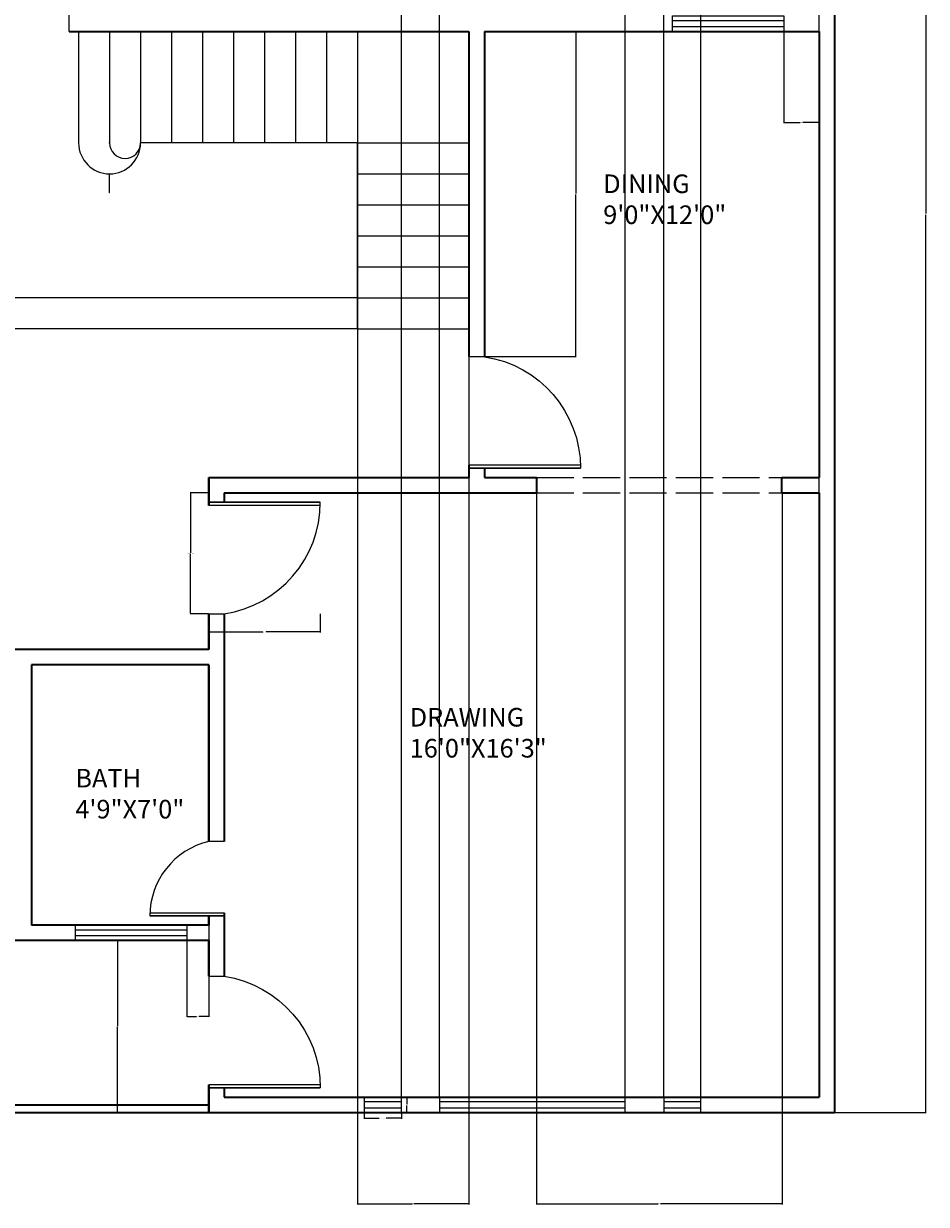
# Model space of a CAD drawing. Units: inches. Extents: x 40921 to 41493, y 89872 to 90511.
# Tile 3 of 4: x 41201 to 41493, y 89872 to 90253. Entities that reach past the tile are written whole.
import ezdxf

# ---------------------------------------------------------------- set-up
doc = ezdxf.new("R2010")
doc.units = ezdxf.units.IN
doc.header["$MEASUREMENT"] = 0
doc.linetypes.add('ACAD_ISO02W100', pattern=[15, 12, -3])
for name, color, linetype, lineweight in [('A-ANNO-DIMS', 2, 'Continuous', 18), ('A-AREA-IDEN', 7, 'Continuous', 18), ('A-DOOR', 3, 'Continuous', 20), ('A-FLOR-STRS', 7, 'Continuous', 18), ('A-GLAZ', 4, 'Continuous', 18), ('A-WALL', 7, 'Continuous', 35), ('A-WALL-OVHD', 8, 'ACAD_ISO02W100', 13)]:
    doc.layers.add(name, color=color, linetype=linetype, lineweight=lineweight)
doc.styles.get("Standard").update_dxf_attribs({"font": 'arial.ttf'})
doc.dimstyles.get("Standard").update_dxf_attribs({"dimtxt": 0.18, "dimasz": 0.18, "dimexe": 0.18, "dimexo": 0.0625, "dimgap": 0.09, "dimtad": 0, "dimtih": 1, "dimtoh": 1, "dimdec": 4, "dimzin": 0, "dimdsep": 46, "dimtxsty": 'Standard', "dimcen": 0.09, "dimadec": 0, "dimazin": 0, "dimtfac": 1, "dimtdec": 4, "dimtofl": 0, "dimtmove": 0, "dimatfit": 3, "dimfxl": 1, "dimtolj": 1, "dimtzin": 0, "dimarcsym": 0})

# ---------------------------------------------------------------- blocks, each defined once
blk = doc.blocks.new('DOOR-SWING-24IN')
for p, q in [((3, 0), (3, 24)), ((3, 24), (3, 0)), ((4, 24), (4, 0)), ((27, 0), (27, 5)), ((0, 0), (3, 0)), ((3, 0), (4, 0))]:
    blk.add_line(p, q)
blk.add_arc((3, -0.66), 24.66, 13.265, 90)
blk = doc.blocks.new('DOOR-SWING-36IN')
for p, q in [((3, 0), (3, 36)), ((3, 36), (3, 0)), ((4, 36), (4, 0)), ((39, 0), (39, 5)), ((0, 0), (3, 0)), ((3, 0), (4, 0))]:
    blk.add_line(p, q)
blk.add_arc((3, -0.4), 36.4, 8.5358, 90)
blk = doc.blocks.new('WIN-36IN')
for p, q in [((0, 36), (5, 36)), ((0, 0), (0, 36)), ((1.5, 0), (1.5, 36)), ((3.5, 36), (3.5, 0)), ((5, 36), (5, 0)), ((5, 0), (0, 0))]:
    blk.add_line(p, q)
blk = doc.blocks.new('WIN-60IN')
for p, q in [((0, 5), (0, 0)), ((60, 5), (0, 5)), ((60, 0), (60, 5)), ((60, 3.5), (0, 3.5)), ((0, 1.5), (60, 1.5)), ((0, 0), (60, 0))]:
    blk.add_line(p, q)
blk = doc.blocks.new('WIN-12IN')
for p, q in [((0, 5), (0, 0)), ((12, 5), (0, 5)), ((12, 0), (12, 5)), ((12, 3.5), (0, 3.5)), ((0, 1.5), (12, 1.5)), ((0, 0), (12, 0))]:
    blk.add_line(p, q)
blk = doc.blocks.new('*D11')
at = {"layer": 'A-ANNO-DIMS', "color": 0, "lineweight": -2, "transparency": 16777216}
for p, q in [((41311.33, 89901.57), (41311.33, 89899.65)), ((41323.33, 89901.57), (41323.33, 89899.65)), ((41311.51, 89899.83), (41316.21, 89899.83)), ((41323.15, 89899.83), (41318.45, 89899.83))]:
    blk.add_line(p, q, dxfattribs=at)
at = {"layer": 'A-ANNO-DIMS', "color": 0, "transparency": 16777216}
for points in [[(41311.51, 89899.86), (41311.51, 89899.8), (41311.33, 89899.83)], [(41323.15, 89899.86), (41323.15, 89899.8), (41323.33, 89899.83)]]:
    blk.add_solid(points, dxfattribs=at)
at = {"layer": 'Defpoints', "color": 0, "transparency": 16777216}
for p in [(41311.33, 89901.63), (41323.33, 89901.63), (41323.33, 89899.83)]:
    blk.add_point(p, dxfattribs=at)
at = {"layer": 'A-ANNO-DIMS', "color": 0, "transparency": 16777216, "insert": (41317.33, 89899.83), "char_height": 0.18, "attachment_point": 5}
blk.add_mtext('\\A1;WINDOW 12 TYP.', dxfattribs=at)
blk = doc.blocks.new('*D12')
at = {"layer": 'A-ANNO-DIMS', "color": 0, "lineweight": -2, "transparency": 16777216}
for p, q in [((41323.39, 89906.63), (41325.31, 89906.63)), ((41325.13, 89906.45), (41325.13, 89904.31)), ((41323.39, 89901.63), (41325.31, 89901.63)), ((41325.13, 89901.81), (41325.13, 89903.95))]:
    blk.add_line(p, q, dxfattribs=at)
at = {"layer": 'A-ANNO-DIMS', "color": 0, "transparency": 16777216}
for points in [[(41325.1, 89906.45), (41325.16, 89906.45), (41325.13, 89906.63)], [(41325.1, 89901.81), (41325.16, 89901.81), (41325.13, 89901.63)]]:
    blk.add_solid(points, dxfattribs=at)
at = {"layer": 'Defpoints', "color": 0, "transparency": 16777216}
for p in [(41323.33, 89906.63), (41325.13, 89906.63), (41323.33, 89901.63)]:
    blk.add_point(p, dxfattribs=at)
at = {"layer": 'A-ANNO-DIMS', "color": 0, "transparency": 16777216, "insert": (41325.13, 89904.13), "char_height": 0.18, "attachment_point": 5}
blk.add_mtext('\\A1;5 TYP.', dxfattribs=at)
blk = doc.blocks.new('*D15')
at = {"layer": 'A-ANNO-DIMS', "color": 0, "lineweight": -2, "transparency": 16777216}
for p, q in [((41261.09, 90101.63), (41255.12, 90101.63)), ((41255.3, 90101.45), (41255.3, 90082.31)), ((41255.3, 90062.81), (41255.3, 90081.95)), ((41261.09, 90062.63), (41255.12, 90062.63))]:
    blk.add_line(p, q, dxfattribs=at)
at = {"layer": 'A-ANNO-DIMS', "color": 0, "transparency": 16777216}
for points in [[(41255.27, 90101.45), (41255.33, 90101.45), (41255.3, 90101.63)], [(41255.27, 90062.81), (41255.33, 90062.81), (41255.3, 90062.63)]]:
    blk.add_solid(points, dxfattribs=at)
at = {"layer": 'Defpoints', "color": 0, "transparency": 16777216}
for p in [(41261.15, 90101.63), (41255.3, 90062.63), (41261.15, 90062.63)]:
    blk.add_point(p, dxfattribs=at)
at = {"layer": 'A-ANNO-DIMS', "color": 0, "transparency": 16777216, "insert": (41255.3, 90082.13), "char_height": 0.18, "attachment_point": 5}
blk.add_mtext('\\A1;ROOM DOOR 39 TYP.', dxfattribs=at)
blk = doc.blocks.new('*D16')
at = {"layer": 'A-ANNO-DIMS', "color": 0, "lineweight": -2, "transparency": 16777216}
for p, q in [((41261.15, 90062.57), (41261.15, 90056.6)), ((41297.15, 90062.57), (41297.15, 90056.6)), ((41261.33, 90056.78), (41278.62, 90056.78)), ((41296.97, 90056.78), (41279.68, 90056.78))]:
    blk.add_line(p, q, dxfattribs=at)
at = {"layer": 'A-ANNO-DIMS', "color": 0, "transparency": 16777216}
for points in [[(41261.33, 90056.81), (41261.33, 90056.75), (41261.15, 90056.78)], [(41296.97, 90056.81), (41296.97, 90056.75), (41297.15, 90056.78)]]:
    blk.add_solid(points, dxfattribs=at)
at = {"layer": 'Defpoints', "color": 0, "transparency": 16777216}
for p in [(41261.15, 90062.63), (41297.15, 90062.63), (41297.15, 90056.78)]:
    blk.add_point(p, dxfattribs=at)
at = {"layer": 'A-ANNO-DIMS', "color": 0, "transparency": 16777216, "insert": (41279.15, 90056.78), "char_height": 0.18, "attachment_point": 5}
blk.add_mtext('\\A1;36 TYP.', dxfattribs=at)
blk = doc.blocks.new('*D20')
at = {"layer": 'A-ANNO-DIMS', "color": 0, "lineweight": -2, "transparency": 16777216}
for p, q in [((41463.21, 90481.63), (41492.78, 90481.63)), ((41492.6, 90481.45), (41492.6, 90191.81)), ((41492.6, 89901.81), (41492.6, 90191.45)), ((41463.21, 89901.63), (41492.78, 89901.63))]:
    blk.add_line(p, q, dxfattribs=at)
at = {"layer": 'A-ANNO-DIMS', "color": 0, "transparency": 16777216}
for points in [[(41492.57, 90481.45), (41492.63, 90481.45), (41492.6, 90481.63)], [(41492.57, 89901.81), (41492.63, 89901.81), (41492.6, 89901.63)]]:
    blk.add_solid(points, dxfattribs=at)
at = {"layer": 'Defpoints', "color": 0, "transparency": 16777216}
for p in [(41463.15, 90481.63), (41492.6, 90481.63), (41463.15, 89901.63)]:
    blk.add_point(p, dxfattribs=at)
at = {"layer": 'A-ANNO-DIMS', "color": 0, "transparency": 16777216, "insert": (41492.6, 90191.63), "char_height": 0.18, "attachment_point": 5}
blk.add_mtext('\\A1;580', dxfattribs=at)
blk = doc.blocks.new('*D24')
at = {"layer": 'A-ANNO-DIMS', "color": 0, "lineweight": -2, "transparency": 16777216}
for p, q in [((41261.09, 89957.13), (41231.52, 89957.13)), ((41231.7, 89956.95), (41231.7, 89929.56)), ((41231.7, 89901.81), (41231.7, 89929.2)), ((41261.09, 89901.63), (41231.52, 89901.63))]:
    blk.add_line(p, q, dxfattribs=at)
at = {"layer": 'A-ANNO-DIMS', "color": 0, "transparency": 16777216}
for points in [[(41231.67, 89956.95), (41231.73, 89956.95), (41231.7, 89957.13)], [(41231.67, 89901.81), (41231.73, 89901.81), (41231.7, 89901.63)]]:
    blk.add_solid(points, dxfattribs=at)
at = {"layer": 'Defpoints', "color": 0, "transparency": 16777216}
for p in [(41231.7, 89957.13), (41261.15, 89957.13), (41261.15, 89901.63)]:
    blk.add_point(p, dxfattribs=at)
at = {"layer": 'A-ANNO-DIMS', "color": 0, "transparency": 16777216, "insert": (41231.7, 89929.38), "char_height": 0.18, "attachment_point": 5}
blk.add_mtext('\\A1;55.5', dxfattribs=at)
blk = doc.blocks.new('*D27')
at = {"layer": 'A-ANNO-DIMS', "color": 0, "lineweight": -2, "transparency": 16777216}
for p, q in [((41309.15, 90154.57), (41309.15, 89872)), ((41345.15, 90154.57), (41345.15, 89872)), ((41309.33, 89872.18), (41326.93, 89872.18)), ((41344.97, 89872.18), (41327.37, 89872.18))]:
    blk.add_line(p, q, dxfattribs=at)
at = {"layer": 'A-ANNO-DIMS', "color": 0, "transparency": 16777216}
for points in [[(41309.33, 89872.21), (41309.33, 89872.15), (41309.15, 89872.18)], [(41344.97, 89872.21), (41344.97, 89872.15), (41345.15, 89872.18)]]:
    blk.add_solid(points, dxfattribs=at)
at = {"layer": 'Defpoints', "color": 0, "transparency": 16777216}
for p in [(41309.15, 90154.63), (41345.15, 90154.63), (41345.15, 89872.18)]:
    blk.add_point(p, dxfattribs=at)
at = {"layer": 'A-ANNO-DIMS', "color": 0, "transparency": 16777216, "insert": (41327.15, 89872.18), "char_height": 0.18, "attachment_point": 5}
blk.add_mtext('\\A1;36', dxfattribs=at)
blk = doc.blocks.new('*D28')
at = {"layer": 'A-ANNO-DIMS', "color": 0, "lineweight": -2, "transparency": 16777216}
for p, q in [((41309.09, 90164.63), (40921.52, 90164.63)), ((40921.7, 90164.45), (40921.7, 90159.81)), ((40921.7, 90154.81), (40921.7, 90159.45)), ((41309.09, 90154.63), (40921.52, 90154.63))]:
    blk.add_line(p, q, dxfattribs=at)
at = {"layer": 'A-ANNO-DIMS', "color": 0, "transparency": 16777216}
for points in [[(40921.67, 90164.45), (40921.73, 90164.45), (40921.7, 90164.63)], [(40921.67, 90154.81), (40921.73, 90154.81), (40921.7, 90154.63)]]:
    blk.add_solid(points, dxfattribs=at)
at = {"layer": 'Defpoints', "color": 0, "transparency": 16777216}
for p in [(40921.7, 90164.63), (41309.15, 90164.63), (41309.15, 90154.63)]:
    blk.add_point(p, dxfattribs=at)
at = {"layer": 'A-ANNO-DIMS', "color": 0, "transparency": 16777216, "insert": (40921.7, 90159.63), "char_height": 0.18, "attachment_point": 5}
blk.add_mtext('\\A1;10', dxfattribs=at)
blk = doc.blocks.new('*D29')
at = {"layer": 'A-ANNO-DIMS', "color": 0, "lineweight": -2, "transparency": 16777216}
for p, q in [((41366.95, 90101.57), (41366.95, 89872)), ((41446.2, 90101.57), (41446.2, 89872)), ((41367.13, 89872.18), (41406.18, 89872.18)), ((41446.02, 89872.18), (41406.97, 89872.18))]:
    blk.add_line(p, q, dxfattribs=at)
at = {"layer": 'A-ANNO-DIMS', "color": 0, "transparency": 16777216}
for points in [[(41367.13, 89872.21), (41367.13, 89872.15), (41366.95, 89872.18)], [(41446.02, 89872.21), (41446.02, 89872.15), (41446.2, 89872.18)]]:
    blk.add_solid(points, dxfattribs=at)
at = {"layer": 'Defpoints', "color": 0, "transparency": 16777216}
for p in [(41366.95, 90101.63), (41446.2, 90101.63), (41446.2, 89872.18)]:
    blk.add_point(p, dxfattribs=at)
at = {"layer": 'A-ANNO-DIMS', "color": 0, "transparency": 16777216, "insert": (41406.57, 89872.18), "char_height": 0.18, "attachment_point": 5}
blk.add_mtext('\\A1;79.24', dxfattribs=at)
blk = doc.blocks.new('*D31')
at = {"layer": 'A-ANNO-DIMS', "color": 0, "lineweight": -2, "transparency": 16777216}
for p, q in [((41420.03, 89906.69), (41420.03, 90511.26)), ((41420.21, 90511.08), (41438.7, 90511.08)), ((41457.97, 90511.08), (41439.48, 90511.08)), ((41458.15, 89906.69), (41458.15, 90511.26))]:
    blk.add_line(p, q, dxfattribs=at)
at = {"layer": 'A-ANNO-DIMS', "color": 0, "transparency": 16777216}
for points in [[(41420.21, 90511.11), (41420.21, 90511.05), (41420.03, 90511.08)], [(41457.97, 90511.11), (41457.97, 90511.05), (41458.15, 90511.08)]]:
    blk.add_solid(points, dxfattribs=at)
at = {"layer": 'Defpoints', "color": 0, "transparency": 16777216}
for p in [(41458.15, 90511.08), (41420.03, 89906.63), (41458.15, 89906.63)]:
    blk.add_point(p, dxfattribs=at)
at = {"layer": 'A-ANNO-DIMS', "color": 0, "transparency": 16777216, "insert": (41439.09, 90511.08), "char_height": 0.18, "attachment_point": 5}
blk.add_mtext('\\A1;38.12', dxfattribs=at)
blk = doc.blocks.new('*D32')
at = {"layer": 'A-ANNO-DIMS', "color": 0, "lineweight": -2, "transparency": 16777216}
for p, q in [((41323.33, 89906.69), (41323.33, 90511.26)), ((41323.51, 90511.08), (41329.01, 90511.08)), ((41335.42, 90511.08), (41329.92, 90511.08)), ((41335.6, 89906.69), (41335.6, 90511.26))]:
    blk.add_line(p, q, dxfattribs=at)
at = {"layer": 'A-ANNO-DIMS', "color": 0, "transparency": 16777216}
for points in [[(41323.51, 90511.11), (41323.51, 90511.05), (41323.33, 90511.08)], [(41335.42, 90511.11), (41335.42, 90511.05), (41335.6, 90511.08)]]:
    blk.add_solid(points, dxfattribs=at)
at = {"layer": 'Defpoints', "color": 0, "transparency": 16777216}
for p in [(41335.6, 90511.08), (41323.33, 89906.63), (41335.6, 89906.63)]:
    blk.add_point(p, dxfattribs=at)
at = {"layer": 'A-ANNO-DIMS', "color": 0, "transparency": 16777216, "insert": (41329.46, 90511.08), "char_height": 0.18, "attachment_point": 5}
blk.add_mtext('\\A1;12.272', dxfattribs=at)
blk = doc.blocks.new('*D33')
at = {"layer": 'A-ANNO-DIMS', "color": 0, "lineweight": -2, "transparency": 16777216}
for p, q in [((41395.6, 89906.69), (41395.6, 90511.26)), ((41395.78, 90511.08), (41401.36, 90511.08)), ((41407.85, 90511.08), (41402.27, 90511.08)), ((41408.03, 89906.69), (41408.03, 90511.26))]:
    blk.add_line(p, q, dxfattribs=at)
at = {"layer": 'A-ANNO-DIMS', "color": 0, "transparency": 16777216}
for points in [[(41395.78, 90511.11), (41395.78, 90511.05), (41395.6, 90511.08)], [(41407.85, 90511.11), (41407.85, 90511.05), (41408.03, 90511.08)]]:
    blk.add_solid(points, dxfattribs=at)
at = {"layer": 'Defpoints', "color": 0, "transparency": 16777216}
for p in [(41408.03, 90511.08), (41395.6, 89906.63), (41408.03, 89906.63)]:
    blk.add_point(p, dxfattribs=at)
at = {"layer": 'A-ANNO-DIMS', "color": 0, "transparency": 16777216, "insert": (41401.81, 90511.08), "char_height": 0.18, "attachment_point": 5}
blk.add_mtext('\\A1;12.429', dxfattribs=at)
blk = doc.blocks.new('*D40')
at = {"layer": 'A-ANNO-DIMS', "color": 0, "lineweight": -2, "transparency": 16777216}
for p, q in [((41350.21, 90250.63), (41379.78, 90250.63)), ((41379.6, 90250.45), (41379.6, 90198.31)), ((41379.6, 90145.81), (41379.6, 90197.95)), ((41350.21, 90145.63), (41379.78, 90145.63))]:
    blk.add_line(p, q, dxfattribs=at)
at = {"layer": 'A-ANNO-DIMS', "color": 0, "transparency": 16777216}
for points in [[(41379.57, 90250.45), (41379.63, 90250.45), (41379.6, 90250.63)], [(41379.57, 90145.81), (41379.63, 90145.81), (41379.6, 90145.63)]]:
    blk.add_solid(points, dxfattribs=at)
at = {"layer": 'Defpoints', "color": 0, "transparency": 16777216}
for p in [(41350.15, 90250.63), (41350.15, 90145.63), (41379.6, 90145.63)]:
    blk.add_point(p, dxfattribs=at)
at = {"layer": 'A-ANNO-DIMS', "color": 0, "transparency": 16777216, "insert": (41379.6, 90198.13), "char_height": 0.18, "attachment_point": 5}
blk.add_mtext('\\A1;105', dxfattribs=at)
blk = doc.blocks.new('*D42')
at = {"layer": 'A-ANNO-DIMS', "color": 0, "lineweight": -2, "transparency": 16777216}
for p, q in [((41254.12, 89962.07), (41254.12, 89932.5)), ((41261.15, 89962.07), (41261.15, 89932.5)), ((41254.3, 89932.68), (41257.24, 89932.68)), ((41260.97, 89932.68), (41258.03, 89932.68))]:
    blk.add_line(p, q, dxfattribs=at)
at = {"layer": 'A-ANNO-DIMS', "color": 0, "transparency": 16777216}
for points in [[(41254.3, 89932.71), (41254.3, 89932.65), (41254.12, 89932.68)], [(41260.97, 89932.71), (41260.97, 89932.65), (41261.15, 89932.68)]]:
    blk.add_solid(points, dxfattribs=at)
at = {"layer": 'Defpoints', "color": 0, "transparency": 16777216}
for p in [(41254.12, 89962.13), (41261.15, 89962.13), (41254.12, 89932.68)]:
    blk.add_point(p, dxfattribs=at)
at = {"layer": 'A-ANNO-DIMS', "color": 0, "transparency": 16777216, "insert": (41257.63, 89932.68), "char_height": 0.18, "attachment_point": 5}
blk.add_mtext('\\A1;7.032', dxfattribs=at)
blk = doc.blocks.new('*D44')
at = {"layer": 'A-ANNO-DIMS', "color": 0, "lineweight": -2, "transparency": 16777216}
for p, q in [((41446.81, 90250.57), (41446.81, 90221)), ((41458.15, 90250.57), (41458.15, 90221)), ((41446.99, 90221.18), (41452.1, 90221.18)), ((41457.97, 90221.18), (41452.87, 90221.18))]:
    blk.add_line(p, q, dxfattribs=at)
at = {"layer": 'A-ANNO-DIMS', "color": 0, "transparency": 16777216}
for points in [[(41446.99, 90221.21), (41446.99, 90221.15), (41446.81, 90221.18)], [(41457.97, 90221.21), (41457.97, 90221.15), (41458.15, 90221.18)]]:
    blk.add_solid(points, dxfattribs=at)
at = {"layer": 'Defpoints', "color": 0, "transparency": 16777216}
for p in [(41446.81, 90250.63), (41458.15, 90250.63), (41446.81, 90221.18)]:
    blk.add_point(p, dxfattribs=at)
at = {"layer": 'A-ANNO-DIMS', "color": 0, "transparency": 16777216, "insert": (41452.48, 90221.18), "char_height": 0.18, "attachment_point": 5}
blk.add_mtext('\\A1;11.34', dxfattribs=at)
blk = doc.blocks.new('*D46')
at = {"layer": 'A-ANNO-DIMS', "color": 0, "lineweight": -2, "transparency": 16777216}
for p, q in [((41218.16, 90294.36), (41204.02, 90277.95)), ((41218.34, 90294.36), (41218.16, 90294.36)), ((41180.06, 90250.23), (41180.24, 90250.23)), ((41180.15, 90250.14), (41180.15, 90250.32))]:
    blk.add_line(p, q, dxfattribs=at)
at = {"layer": 'A-ANNO-DIMS', "color": 0, "transparency": 16777216}
blk.add_solid([(41204, 90277.97), (41204.04, 90277.93), (41203.9, 90277.81)], dxfattribs=at)
at = {"layer": 'Defpoints', "color": 0, "transparency": 16777216}
for p in [(41203.9, 90277.81), (41180.15, 90250.23)]:
    blk.add_point(p, dxfattribs=at)
at = {"layer": 'A-ANNO-DIMS', "color": 0, "transparency": 16777216, "insert": (41218.94, 90294.36), "char_height": 0.18, "attachment_point": 5}
blk.add_mtext('\\A1;2X R36.4', dxfattribs=at)
blk = doc.blocks.new('*D50')
at = {"layer": 'A-ANNO-DIMS', "color": 0, "lineweight": -2, "transparency": 16777216}
for p, q in [((41229.06, 90214.63), (41229.24, 90214.63)), ((41229.15, 90214.54), (41229.15, 90214.72)), ((41229.15, 90198.63), (41229.15, 90204.45)), ((41228.97, 90198.63), (41229.15, 90198.63))]:
    blk.add_line(p, q, dxfattribs=at)
at = {"layer": 'A-ANNO-DIMS', "color": 0, "transparency": 16777216}
blk.add_solid([(41229.12, 90204.45), (41229.18, 90204.45), (41229.15, 90204.63)], dxfattribs=at)
at = {"layer": 'Defpoints', "color": 0, "transparency": 16777216}
for p in [(41229.15, 90214.63), (41229.15, 90204.63)]:
    blk.add_point(p, dxfattribs=at)
at = {"layer": 'A-ANNO-DIMS', "color": 0, "transparency": 16777216, "insert": (41228.67, 90198.63), "char_height": 0.18, "attachment_point": 5}
blk.add_mtext('\\A1;R10', dxfattribs=at)

msp = doc.modelspace()

# ---------------------------------------------------------------- linework, layer by layer
at = {"layer": 'A-FLOR-STRS'}
for p, q in [((41219.1503, 90250.6306), (41219.1503, 90214.6306)), ((41229.1503, 90250.6306), (41229.1503, 90214.6306)), ((41239.1503, 90250.6306), (41239.1503, 90214.6306)), ((41249.1503, 90250.6306), (41249.1503, 90214.6306)), ((41259.1503, 90250.6306), (41259.1503, 90214.6306)), ((41269.1503, 90250.6306), (41269.1503, 90214.6306)), ((41279.1503, 90250.6306), (41279.1503, 90214.6306)), ((41289.1503, 90250.6306), (41289.1503, 90214.6306)), ((41299.1503, 90250.6306), (41299.1503, 90214.6306)), ((41345.1503, 90250.6306), (41309.1503, 90250.6306)), ((41309.1503, 90250.6306), (41309.1503, 90214.6306)), ((41309.1503, 90214.6306), (41239.1503, 90214.6306)), ((41309.1503, 90214.6306), (41345.1503, 90214.6306)), ((41309.1503, 90214.6306), (41309.1503, 90154.6306)), ((41309.1503, 90154.6306), (41309.1503, 90214.6306)), ((41309.1503, 90204.6306), (41345.1503, 90204.6306)), ((41309.1503, 90194.6306), (41345.1503, 90194.6306)), ((41309.1503, 90184.6306), (41345.1503, 90184.6306)), ((41309.1503, 90174.6306), (41345.1503, 90174.6306)), ((41309.1503, 90164.6306), (41345.1503, 90164.6306)), ((41309.1503, 90154.6306), (41345.1503, 90154.6306))]:
    msp.add_line(p, q, dxfattribs=at)
for centre, radius in [((41229.1503, 90214.6306), 10), ((41234.1503, 90214.6306), 5)]:
    msp.add_arc(centre, radius, 180, 0, dxfattribs=at)
at = {"layer": 'A-WALL'}
for p, q in [((41463.1503, 90481.6306), (41463.1503, 89901.6306)), ((41216.1503, 90250.6306), (41345.1503, 90250.6306)), ((41345.1503, 90250.6306), (41345.1503, 90145.6306)), ((41350.1503, 90250.6306), (41350.1503, 90145.6306)), ((41350.1503, 90250.6306), (41458.1503, 90250.6306)), ((41458.1503, 90250.6306), (41458.1503, 90106.6306)), ((41345.1503, 90110.6306), (41345.1503, 90106.6306)), ((41350.1503, 90109.6306), (41350.1503, 90106.6306)), ((41261.1503, 90106.6306), (41261.1503, 90097.6306)), ((41261.1503, 90106.6306), (41345.1503, 90106.6306)), ((41261.1503, 90097.6306), (41261.1503, 90106.6306)), ((41350.1503, 90106.6306), (41366.9523, 90106.6306)), ((41366.9523, 90106.6306), (41366.9523, 90101.6306)), ((41446.1963, 90101.6306), (41446.1963, 90106.6306)), ((41446.1963, 90106.6306), (41458.1503, 90106.6306)), ((41266.1503, 90101.6306), (41266.1503, 90098.6306)), ((41266.1503, 90101.6306), (41366.9523, 90101.6306)), ((41446.1963, 90101.6306), (41458.1503, 90101.6306)), ((41458.1503, 90101.6306), (41458.1503, 89906.6306)), ((41261.1503, 90062.6306), (41261.1503, 90051.1306)), ((41261.1503, 90051.1306), (41261.1503, 90062.6306)), ((41266.1503, 90062.6306), (41266.1503, 89989.1306)), ((41261.1503, 90051.1306), (41194.9003, 90051.1306)), ((41261.1503, 90046.1306), (41203.9003, 90046.1306)), ((41203.9003, 90046.1306), (41203.9003, 89962.1306)), ((41261.1503, 89989.1306), (41261.1503, 90046.1306)), ((41261.1503, 90046.1306), (41261.1503, 89989.1306)), ((41266.1503, 89966.1306), (41266.1503, 89945.6306)), ((41261.1503, 89962.1306), (41203.9003, 89962.1306)), ((41261.1503, 89965.1306), (41261.1503, 89962.1306)), ((41261.1503, 89962.1306), (41261.1503, 89965.1306)), ((41261.1503, 89957.1306), (41136.6503, 89957.1306)), ((41261.1503, 89945.6306), (41261.1503, 89957.1306)), ((41261.1503, 89957.1306), (41261.1503, 89945.6306)), ((41261.1503, 89901.6306), (41261.1503, 89910.6306)), ((41261.1503, 89910.6306), (41261.1503, 89901.6306)), ((41266.1503, 89909.6306), (41266.1503, 89906.6306)), ((41266.1503, 89906.6306), (41458.1503, 89906.6306)), ((41114.6387, 89901.6306), (41463.1503, 89901.6306)), ((41127.0765, 89904.1306), (41261.1503, 89904.1306))]:
    msp.add_line(p, q, dxfattribs=at)
at = {"layer": 'A-WALL-OVHD'}
for p, q in [((41366.9523, 90106.6306), (41446.1963, 90106.6306)), ((41366.9523, 90101.6306), (41366.9523, 90101.6306)), ((41366.9523, 90101.6306), (41446.1963, 90101.6306))]:
    msp.add_line(p, q, dxfattribs=at)

# ---------------------------------------------------------------- block references
at = {"layer": 'A-DOOR'}
msp.add_blockref('DOOR-SWING-36IN', (41177.15, 90250.631), dxfattribs=at)
at = {"layer": 'A-DOOR', "extrusion": (0, 0, -1), "zscale": -1, "rotation": 89.99999999998715}
for p in [(-41345.1507, 90106.6303), (-41261.1507, 89906.6303)]:
    msp.add_blockref('DOOR-SWING-36IN', p, dxfattribs=at)
at = {"layer": 'A-DOOR'}
for name, p, rotation in [('DOOR-SWING-36IN', (41261.1507, 90101.6309), 270), ('DOOR-SWING-24IN', (41266.1499, 89962.1303), 89.99999999998086)]:
    msp.add_blockref(name, p, dxfattribs=dict(at, rotation=rotation))
at = {"layer": 'A-GLAZ'}
for p, rotation in [((41446.8101, 90250.6303), 89.99999999999685), ((41254.1182, 89957.1303), 90.00000000000003)]:
    msp.add_blockref('WIN-36IN', p, dxfattribs=dict(at, rotation=rotation))
for name, p in [('WIN-12IN', (41311.327, 89901.631)), ('WIN-60IN', (41335.6, 89901.631)), ('WIN-12IN', (41408.0279, 89901.631))]:
    msp.add_blockref(name, p, dxfattribs=at)

# ---------------------------------------------------------------- texts
at = {"layer": 'A-AREA-IDEN', "char_height": 6, "attachment_point": 1}
for s, width, insert in [('DINING\\P9\'0"X12\'0"', 60.330706, (41388.4852, 90204.4377)), ('DRAWING\\P16\'0"X16\'3"', 100.256155, (41326.0144, 90032.2351)), ('BATH\\P4\'9"X7\'0"', 38.908323, (41218.0952, 90012.5714))]:
    msp.add_mtext_dynamic_manual_height_columns(s, width=width, gutter_width=1, heights=[0], dxfattribs=dict(at, insert=insert))

# ---------------------------------------------------------------- dimensions: what is measured, and where the dimension line sits
at = {"layer": 'A-ANNO-DIMS'}
for base, p1, p2, override, picture, middle in [((41335.5998, 90511.0806), (41323.3274, 89906.6306), (41335.5998, 89906.6306), {"dimdec": 3, "dimlfac": 1, "dimrnd": 0, "dimzin": 0, "dimdsep": 46, "dimlunit": 2}, '*D32', (41329.4636, 90511.0806)), ((41408.028255, 90511.080628), (41395.599751, 89906.630628), (41408.028255, 89906.630628), {"dimdec": 3, "dimlfac": 1, "dimrnd": 0, "dimzin": 0, "dimdsep": 46, "dimlunit": 2}, '*D33', (41401.814003, 90511.080628)), ((41458.1503, 90511.0806), (41420.0283, 89906.6306), (41458.1503, 89906.6306), {"dimdec": 2, "dimlfac": 1, "dimrnd": 0, "dimzin": 0, "dimdsep": 46, "dimlunit": 2}, '*D31', (41439.0893, 90511.0806)), ((41345.1503, 89872.1806), (41309.1503, 90154.6306), (41345.1503, 90154.6306), {"dimdec": 0, "dimlfac": 1, "dimrnd": 0, "dimzin": 0, "dimdsep": 46, "dimlunit": 2}, '*D27', (41327.1503, 89872.1806)), ((41446.1963, 89872.1806), (41366.9523, 90101.6306), (41446.1963, 90101.6306), {"dimdec": 2, "dimlfac": 1, "dimrnd": 0, "dimzin": 0, "dimdsep": 46, "dimlunit": 2}, '*D29', (41406.5743, 89872.1806))]:
    dim = msp.add_linear_dim(base=base, p1=p1, p2=p2, dimstyle='Standard', override=override, dxfattribs=at)
    dim.commit()
    dim.dimension.update_dxf_attribs({"geometry": picture, "text_midpoint": middle})
for base, p1, p2, angle, override, picture, middle in [((41492.6003, 90481.6306), (41463.1503, 89901.6306), (41463.1503, 90481.6306), 90, {"dimdec": 0, "dimlfac": 1, "dimrnd": 0, "dimzin": 0, "dimdsep": 46, "dimlunit": 2}, '*D20', (41492.6003, 90191.6306)), ((41379.6003, 90145.6306), (41350.1503, 90250.6306), (41350.1503, 90145.6306), 270, {"dimdec": 0, "dimlfac": 1, "dimrnd": 0, "dimzin": 0, "dimdsep": 46, "dimlunit": 2}, '*D40', (41379.6003, 90198.1306)), ((41446.8104, 90221.1806), (41458.1503, 90250.6306), (41446.8104, 90250.6306), 180, {"dimdec": 2, "dimlfac": 1, "dimrnd": 0, "dimzin": 0, "dimdsep": 46, "dimlunit": 2}, '*D44', (41452.4804, 90221.1806)), ((40921.7003, 90164.6306), (41309.1503, 90154.6306), (41309.1503, 90164.6306), 90, {"dimdec": 0, "dimlfac": 1, "dimrnd": 0, "dimzin": 0, "dimdsep": 46, "dimlunit": 2}, '*D28', (40921.7003, 90159.6306)), ((41254.1186, 89932.6806), (41261.1503, 89962.1306), (41254.1186, 89962.1306), 180, {"dimdec": 3, "dimlfac": 1, "dimrnd": 0, "dimzin": 0, "dimdsep": 46, "dimlunit": 2}, '*D42', (41257.6344, 89932.6806)), ((41231.7003, 89957.1306), (41261.1503, 89901.6306), (41261.1503, 89957.1306), 90, {"dimdec": 1, "dimlfac": 1, "dimrnd": 0, "dimzin": 0, "dimdsep": 46, "dimlunit": 2}, '*D24', (41231.7003, 89929.3806))]:
    dim = msp.add_linear_dim(base=base, p1=p1, p2=p2, angle=angle, dimstyle='Standard', override=override, dxfattribs=at)
    dim.commit()
    dim.dimension.update_dxf_attribs({"geometry": picture, "text_midpoint": middle})
dim = msp.add_radius_dim(center=(41180.1503, 90250.2274), mpoint=(41203.9039, 90277.8129), text='2X <>', dimstyle='Standard', override={"dimdec": 1, "dimlfac": 1, "dimrnd": 0, "dimzin": 0, "dimdsep": 46, "dimlunit": 2}, dxfattribs=at)
dim.commit()
dim.dimension.update_dxf_attribs({"geometry": '*D46', "text_midpoint": (41218.9406, 90294.3642), "dimtype": 164})
dim = msp.add_radius_dim(center=(41229.1503, 90214.6306), mpoint=(41229.15, 90204.6306), dimstyle='Standard', override={"dimdec": 0, "dimlfac": 1, "dimrnd": 0, "dimzin": 0, "dimdsep": 46, "dimlunit": 2}, dxfattribs=at)
dim.commit()
dim.dimension.update_dxf_attribs({"geometry": '*D50', "text_midpoint": (41228.6651, 90198.6306), "dimtype": 164})
for base, p1, p2, angle, text, picture, middle in [((41255.3003, 90062.6306), (41261.1503, 90101.6306), (41261.1503, 90062.6306), 270, 'ROOM DOOR <> TYP.', '*D15', (41255.3003, 90082.1306)), ((41325.1274, 89906.6306), (41323.3274, 89901.6306), (41323.3274, 89906.6306), 90, '<> TYP.', '*D12', (41325.1274, 89904.1306))]:
    dim = msp.add_linear_dim(base=base, p1=p1, p2=p2, angle=angle, text=text, dimstyle='Standard', override={"dimdec": 0, "dimlfac": 1, "dimrnd": 0, "dimzin": 0, "dimdsep": 46, "dimlunit": 2}, dxfattribs=at)
    dim.commit()
    dim.dimension.update_dxf_attribs({"geometry": picture, "text_midpoint": middle})
for base, p1, p2, text, picture, middle in [((41297.1503, 90056.7806), (41261.1503, 90062.6306), (41297.1503, 90062.6306), '<> TYP.', '*D16', (41279.1503, 90056.7806)), ((41323.3274, 89899.8306), (41311.3274, 89901.6306), (41323.3274, 89901.6306), 'WINDOW <> TYP.', '*D11', (41317.3274, 89899.8306))]:
    dim = msp.add_linear_dim(base=base, p1=p1, p2=p2, text=text, dimstyle='Standard', override={"dimdec": 0, "dimlfac": 1, "dimrnd": 0, "dimzin": 0, "dimdsep": 46, "dimlunit": 2}, dxfattribs=at)
    dim.commit()
    dim.dimension.update_dxf_attribs({"geometry": picture, "text_midpoint": middle})

doc.saveas('drawing.dxf')
